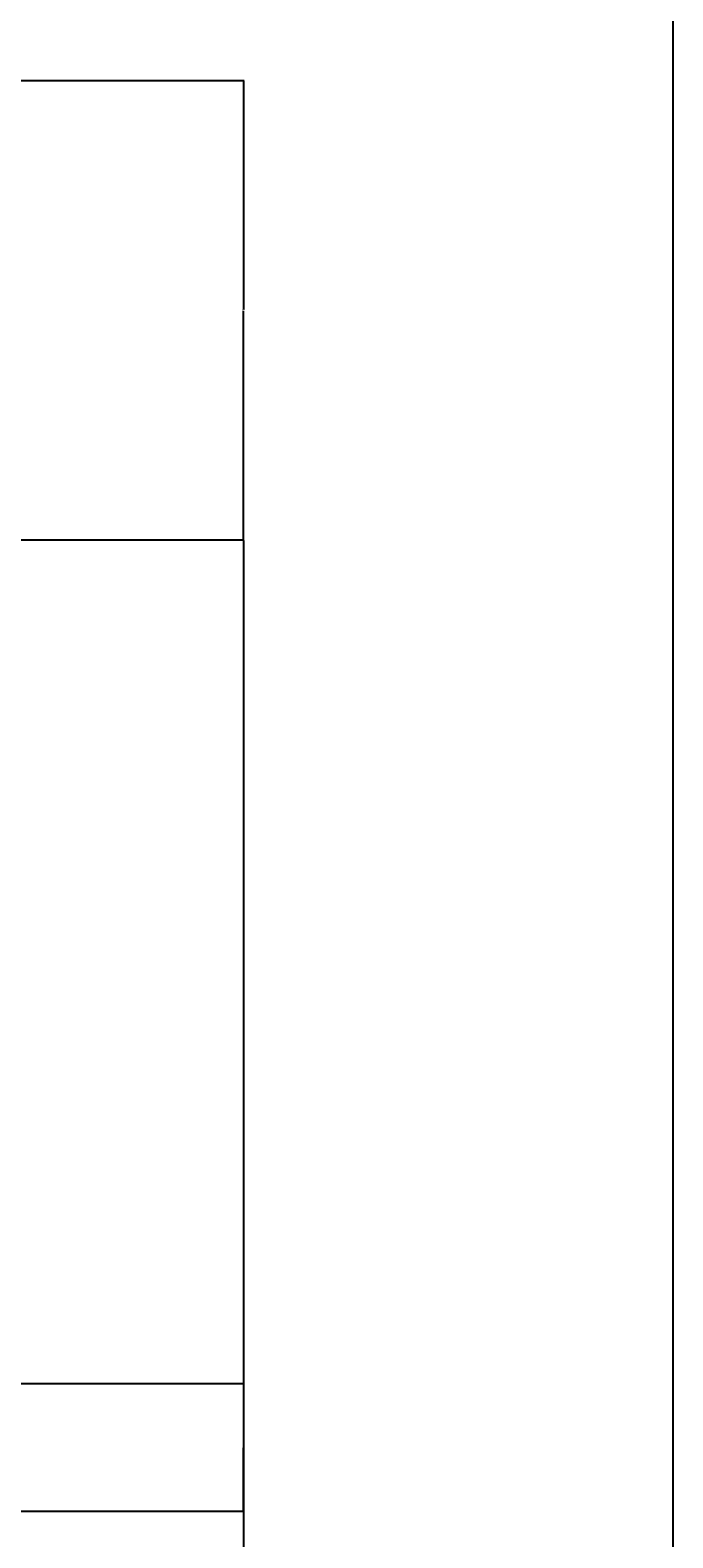
# Model space of a CAD drawing. Units: inches. Extents: x 1770 to 2988, y 1161 to 3221.
# Tile 32 of 44: x 2807 to 2988, y 2095 to 2520. Entities that reach past the tile are written whole.
import ezdxf

# ---------------------------------------------------------------- set-up
doc = ezdxf.new("R2010")
doc.units = ezdxf.units.IN
doc.layers.add('A-ANNO-DIMS', color=2, linetype='Continuous', lineweight=18)
doc.layers.add('A-ANNO-TTLB', color=7, linetype='Continuous', lineweight=25)
doc.styles.get("Standard").update_dxf_attribs({"font": 'arial.ttf'})
doc.dimstyles.get("Standard").update_dxf_attribs({"dimtxt": 0.18, "dimasz": 0.18, "dimexe": 0.18, "dimexo": 0.0625, "dimgap": 0.09, "dimtad": 0, "dimtih": 1, "dimtoh": 1, "dimdec": 4, "dimzin": 0, "dimdsep": 46, "dimtxsty": 'Standard', "dimcen": 0.09, "dimadec": 0, "dimazin": 0, "dimtfac": 1, "dimtdec": 4, "dimtofl": 0, "dimtmove": 0, "dimatfit": 3, "dimfxl": 1, "dimtolj": 1, "dimtzin": 0, "dimarcsym": 0})

# ---------------------------------------------------------------- blocks, each defined once
blk = doc.blocks.new('*D59')
at = {"layer": 'A-ANNO-DIMS', "color": 0, "lineweight": -2, "transparency": 16777216}
for p, q in [((2802.5, 2506.27), (2866.87, 2506.27)), ((2866.69, 2506.09), (2866.69, 2441.67)), ((2866.69, 2376.88), (2866.69, 2441.31)), ((2625.76, 2376.7), (2866.87, 2376.7))]:
    blk.add_line(p, q, dxfattribs=at)
at = {"layer": 'A-ANNO-DIMS', "color": 0, "transparency": 16777216}
for points in [[(2866.66, 2506.09), (2866.72, 2506.09), (2866.69, 2506.27)], [(2866.66, 2376.88), (2866.72, 2376.88), (2866.69, 2376.7)]]:
    blk.add_solid(points, dxfattribs=at)
at = {"layer": 'Defpoints', "color": 0, "transparency": 16777216}
for p in [(2802.44, 2506.27), (2866.69, 2506.27), (2625.7, 2376.7)]:
    blk.add_point(p, dxfattribs=at)
at = {"layer": 'A-ANNO-DIMS', "color": 0, "transparency": 16777216, "insert": (2866.69, 2441.49), "char_height": 0.18, "attachment_point": 5}
blk.add_mtext('\\A1;129.57', dxfattribs=at)
blk = doc.blocks.new('*D61')
at = {"layer": 'A-ANNO-DIMS', "color": 0, "lineweight": -2, "transparency": 16777216}
for p, q in [((2625.76, 2376.7), (2866.87, 2376.7)), ((2866.69, 2376.52), (2866.69, 1993.63)), ((2866.69, 1610.38), (2866.69, 1993.27)), ((2625.76, 1610.2), (2866.87, 1610.2))]:
    blk.add_line(p, q, dxfattribs=at)
at = {"layer": 'A-ANNO-DIMS', "color": 0, "transparency": 16777216}
for points in [[(2866.66, 2376.52), (2866.72, 2376.52), (2866.69, 2376.7)], [(2866.66, 1610.38), (2866.72, 1610.38), (2866.69, 1610.2)]]:
    blk.add_solid(points, dxfattribs=at)
at = {"layer": 'Defpoints', "color": 0, "transparency": 16777216}
for p in [(2625.7, 2376.7), (2866.69, 2376.7), (2625.7, 1610.2)]:
    blk.add_point(p, dxfattribs=at)
at = {"layer": 'A-ANNO-DIMS', "color": 0, "transparency": 16777216, "insert": (2866.69, 1993.45), "char_height": 0.18, "attachment_point": 5}
blk.add_mtext('\\A1;766.5', dxfattribs=at)
blk = doc.blocks.new('*D89')
at = {"layer": 'A-ANNO-DIMS', "color": 0, "lineweight": -2, "transparency": 16777216}
for p, q in [((2160.76, 2138.84), (2866.87, 2138.84)), ((2866.69, 2138.66), (2866.69, 2121.02)), ((2866.69, 2103.02), (2866.69, 2120.66)), ((2160.76, 2102.84), (2866.87, 2102.84))]:
    blk.add_line(p, q, dxfattribs=at)
at = {"layer": 'A-ANNO-DIMS', "color": 0, "transparency": 16777216}
for points in [[(2866.66, 2138.66), (2866.72, 2138.66), (2866.69, 2138.84)], [(2866.66, 2103.02), (2866.72, 2103.02), (2866.69, 2102.84)]]:
    blk.add_solid(points, dxfattribs=at)
at = {"layer": 'Defpoints', "color": 0, "transparency": 16777216}
for p in [(2160.7, 2138.84), (2866.69, 2138.84), (2160.7, 2102.84)]:
    blk.add_point(p, dxfattribs=at)
at = {"layer": 'A-ANNO-DIMS', "color": 0, "transparency": 16777216, "insert": (2866.69, 2120.84), "char_height": 0.18, "attachment_point": 5}
blk.add_mtext('\\A1;36', dxfattribs=at)

msp = doc.modelspace()

# ---------------------------------------------------------------- linework, layer by layer
at = {"layer": 'A-ANNO-TTLB'}
msp.add_lwpolyline([(1769.9155, 3221.2788), (2987.7567, 3221.2788), (2987.7567, 1161.1516), (1769.9155, 1161.1516)], close=True, dxfattribs=at)

# ---------------------------------------------------------------- dimensions: what is measured, and where the dimension line sits
at = {"layer": 'A-ANNO-DIMS'}
for base, p1, p2, override, picture, middle in [((2866.6874, 2506.2747), (2625.696, 2376.7021), (2802.4374, 2506.2747), {"dimdec": 2, "dimlfac": 1, "dimrnd": 0, "dimzin": 0, "dimdsep": 46, "dimlunit": 2}, '*D59', (2866.6874, 2441.4884)), ((2866.6874, 2376.7021), (2625.696, 1610.2021), (2625.696, 2376.7021), {"dimdec": 1, "dimlfac": 1, "dimrnd": 0, "dimzin": 0, "dimdsep": 46, "dimlunit": 2}, '*D61', (2866.6874, 1993.4521)), ((2866.6874, 2138.8392), (2160.696, 2102.8392), (2160.696, 2138.8392), {"dimdec": 0, "dimlfac": 1, "dimrnd": 0, "dimzin": 0, "dimdsep": 46, "dimlunit": 2}, '*D89', (2866.6874, 2120.8392))]:
    dim = msp.add_linear_dim(base=base, p1=p1, p2=p2, angle=90, dimstyle='Standard', override=override, dxfattribs=at)
    dim.commit()
    dim.dimension.update_dxf_attribs({"geometry": picture, "text_midpoint": middle})

doc.saveas('drawing.dxf')
